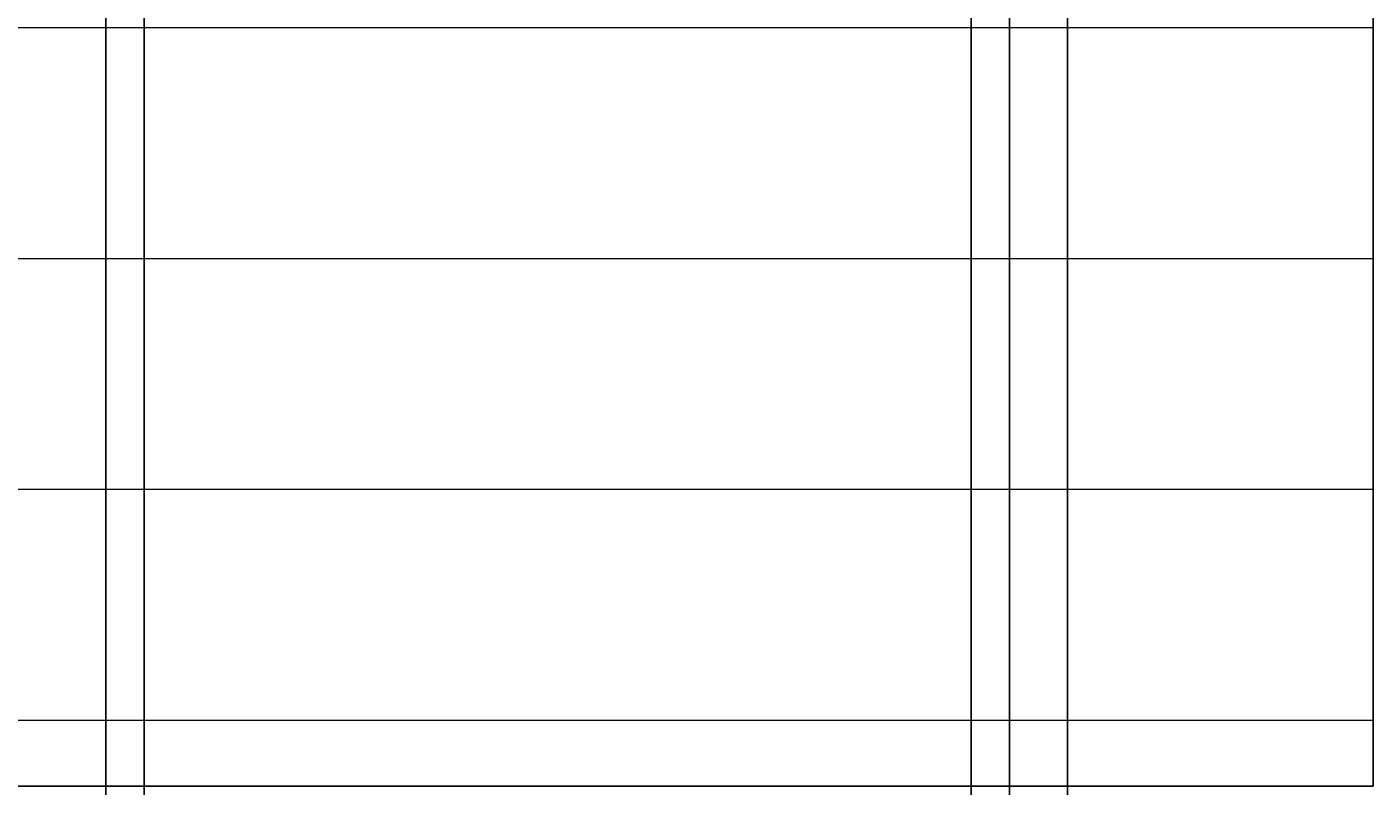
# Model space of a CAD drawing. Units: inches. Extents: x -6 to 289, y -8 to 323.
# Tile 31 of 107: x 209 to 244, y 10 to 30. Entities that reach past the tile are written whole.
import ezdxf

# ---------------------------------------------------------------- set-up
doc = ezdxf.new("R2010")
doc.units = ezdxf.units.IN
doc.header["$MEASUREMENT"] = 0
for name, color, linetype, lineweight in [('A-ANNO-DIMS', 2, 'Continuous', 18), ('A-DOOR', 3, 'Continuous', 25), ('A-ELEV-PATT', 8, 'Continuous', 13)]:
    doc.layers.add(name, color=color, linetype=linetype, lineweight=lineweight)
doc.styles.get("Standard").update_dxf_attribs({"font": 'arial.ttf'})
doc.dimstyles.get("Standard").update_dxf_attribs({"dimtxt": 0.18, "dimasz": 0.18, "dimexe": 0.18, "dimexo": 0.0625, "dimgap": 0.09, "dimtad": 0, "dimtih": 1, "dimtoh": 1, "dimdec": 4, "dimzin": 0, "dimdsep": 46, "dimtxsty": 'Standard', "dimcen": 0.09, "dimadec": 0, "dimazin": 0, "dimtfac": 1, "dimtdec": 4, "dimtofl": 0, "dimtmove": 0, "dimatfit": 3, "dimfxl": 1, "dimtolj": 1, "dimtzin": 0, "dimarcsym": 0})

# ---------------------------------------------------------------- blocks, each defined once
blk = doc.blocks.new('*D16')
at = {"layer": 'A-ANNO-DIMS', "color": 0, "lineweight": -2, "transparency": 16777216}
for p, q in [((9.943, 68.37), (9.943, -8.391)), ((272.973, 68.37), (272.973, -8.391)), ((10.123, -8.211), (140.993, -8.211)), ((272.793, -8.211), (141.923, -8.211))]:
    blk.add_line(p, q, dxfattribs=at)
at = {"layer": 'A-ANNO-DIMS', "color": 0, "transparency": 16777216}
for points in [[(10.123, -8.181), (10.123, -8.241), (9.943, -8.211)], [(272.793, -8.181), (272.793, -8.241), (272.973, -8.211)]]:
    blk.add_solid(points, dxfattribs=at)
at = {"layer": 'Defpoints', "color": 0, "transparency": 16777216}
for p in [(9.943, 68.432), (272.973, 68.432), (272.973, -8.211)]:
    blk.add_point(p, dxfattribs=at)
at = {"layer": 'A-ANNO-DIMS', "color": 0, "transparency": 16777216, "insert": (141.458, -8.211), "char_height": 0.18, "attachment_point": 5}
blk.add_mtext('\\A1;263.03', dxfattribs=at)
blk = doc.blocks.new('*D42')
at = {"layer": 'A-ANNO-DIMS', "color": 0, "lineweight": -2, "transparency": 16777216}
for p, q in [((190.792, 224.326), (190.792, -8.391)), ((211.292, 224.326), (211.292, -8.391)), ((190.972, -8.211), (200.716, -8.211)), ((211.112, -8.211), (201.368, -8.211))]:
    blk.add_line(p, q, dxfattribs=at)
at = {"layer": 'A-ANNO-DIMS', "color": 0, "transparency": 16777216}
for points in [[(190.972, -8.181), (190.972, -8.241), (190.792, -8.211)], [(211.112, -8.181), (211.112, -8.241), (211.292, -8.211)]]:
    blk.add_solid(points, dxfattribs=at)
at = {"layer": 'Defpoints', "color": 0, "transparency": 16777216}
for p in [(190.792, 224.389), (211.292, 224.389), (211.292, -8.211)]:
    blk.add_point(p, dxfattribs=at)
at = {"layer": 'A-ANNO-DIMS', "color": 0, "transparency": 16777216, "insert": (201.042, -8.211), "char_height": 0.18, "attachment_point": 5}
blk.add_mtext('\\A1;20.5', dxfattribs=at)
blk = doc.blocks.new('*D43')
at = {"layer": 'A-ANNO-DIMS', "color": 0, "lineweight": -2, "transparency": 16777216}
for p, q in [((211.292, 224.326), (211.292, -8.391)), ((212.292, 224.326), (212.292, -8.391)), ((211.472, -8.211), (211.669, -8.211)), ((212.112, -8.211), (211.915, -8.211))]:
    blk.add_line(p, q, dxfattribs=at)
at = {"layer": 'A-ANNO-DIMS', "color": 0, "transparency": 16777216}
for points in [[(211.472, -8.181), (211.472, -8.241), (211.292, -8.211)], [(212.112, -8.181), (212.112, -8.241), (212.292, -8.211)]]:
    blk.add_solid(points, dxfattribs=at)
at = {"layer": 'Defpoints', "color": 0, "transparency": 16777216}
for p in [(211.292, 224.389), (212.292, 224.389), (212.292, -8.211)]:
    blk.add_point(p, dxfattribs=at)
at = {"layer": 'A-ANNO-DIMS', "color": 0, "transparency": 16777216, "insert": (211.792, -8.211), "char_height": 0.18, "attachment_point": 5}
blk.add_mtext('\\A1;1', dxfattribs=at)
blk = doc.blocks.new('*D44')
at = {"layer": 'A-ANNO-DIMS', "color": 0, "lineweight": -2, "transparency": 16777216}
for p, q in [((212.292, 224.326), (212.292, -8.391)), ((233.792, 224.326), (233.792, -8.391)), ((212.472, -8.211), (222.716, -8.211)), ((233.612, -8.211), (223.368, -8.211))]:
    blk.add_line(p, q, dxfattribs=at)
at = {"layer": 'A-ANNO-DIMS', "color": 0, "transparency": 16777216}
for points in [[(212.472, -8.181), (212.472, -8.241), (212.292, -8.211)], [(233.612, -8.181), (233.612, -8.241), (233.792, -8.211)]]:
    blk.add_solid(points, dxfattribs=at)
at = {"layer": 'Defpoints', "color": 0, "transparency": 16777216}
for p in [(212.292, 224.389), (233.792, 224.389), (233.792, -8.211)]:
    blk.add_point(p, dxfattribs=at)
at = {"layer": 'A-ANNO-DIMS', "color": 0, "transparency": 16777216, "insert": (223.042, -8.211), "char_height": 0.18, "attachment_point": 5}
blk.add_mtext('\\A1;21.5', dxfattribs=at)
blk = doc.blocks.new('*D45')
at = {"layer": 'A-ANNO-DIMS', "color": 0, "lineweight": -2, "transparency": 16777216}
for p, q in [((234.792, 225.326), (234.792, -8.391)), ((233.792, 224.326), (233.792, -8.391)), ((233.972, -8.211), (234.169, -8.211)), ((234.612, -8.211), (234.415, -8.211))]:
    blk.add_line(p, q, dxfattribs=at)
at = {"layer": 'A-ANNO-DIMS', "color": 0, "transparency": 16777216}
for points in [[(233.972, -8.181), (233.972, -8.241), (233.792, -8.211)], [(234.612, -8.181), (234.612, -8.241), (234.792, -8.211)]]:
    blk.add_solid(points, dxfattribs=at)
at = {"layer": 'Defpoints', "color": 0, "transparency": 16777216}
for p in [(234.792, 225.389), (233.792, 224.389), (234.792, -8.211)]:
    blk.add_point(p, dxfattribs=at)
at = {"layer": 'A-ANNO-DIMS', "color": 0, "transparency": 16777216, "insert": (234.292, -8.211), "char_height": 0.18, "attachment_point": 5}
blk.add_mtext('\\A1;1', dxfattribs=at)
blk = doc.blocks.new('*D46')
at = {"layer": 'A-ANNO-DIMS', "color": 0, "lineweight": -2, "transparency": 16777216}
for p, q in [((236.292, 226.826), (236.292, -8.391)), ((234.792, 225.326), (234.792, -8.391)), ((234.972, -8.211), (235.296, -8.211)), ((236.112, -8.211), (235.788, -8.211))]:
    blk.add_line(p, q, dxfattribs=at)
at = {"layer": 'A-ANNO-DIMS', "color": 0, "transparency": 16777216}
for points in [[(234.972, -8.181), (234.972, -8.241), (234.792, -8.211)], [(236.112, -8.181), (236.112, -8.241), (236.292, -8.211)]]:
    blk.add_solid(points, dxfattribs=at)
at = {"layer": 'Defpoints', "color": 0, "transparency": 16777216}
for p in [(236.292, 226.889), (234.792, 225.389), (236.292, -8.211)]:
    blk.add_point(p, dxfattribs=at)
at = {"layer": 'A-ANNO-DIMS', "color": 0, "transparency": 16777216, "insert": (235.542, -8.211), "char_height": 0.18, "attachment_point": 5}
blk.add_mtext('\\A1;1.5', dxfattribs=at)

msp = doc.modelspace()

# ---------------------------------------------------------------- hatches: boundary and pattern name
at = {"layer": 'A-ELEV-PATT'}
h = msp.add_hatch(dxfattribs=at)
h.set_pattern_fill('_USER', color=256, scale=6, pattern_type=0)
h.set_pattern_definition([(0, (0, 0), (0, 6), [])])
h.paths.add_polyline_path([(184.1244, 48.0851), (124.008, 48.0851), (124.008, 10.2888), (184.1244, 10.2888)])
h.paths.add_polyline_path([(244.2408, 48.0851), (186.3604, 48.0851), (186.3604, 10.2888), (244.2408, 10.2888)])
h.paths.add_polyline_path([(208.2918, 114.2795), (190.7918, 114.2795), (190.7918, 71.2795), (208.2918, 71.2795)])
h.paths.add_polyline_path([(227.7918, 114.2795), (209.2918, 114.2795), (209.2918, 71.2795), (227.7918, 71.2795)])
h.paths.add_polyline_path([(211.2918, 224.3887), (190.7918, 224.3887), (190.7918, 162.3484), (211.2918, 162.3484)])
h.paths.add_polyline_path([(233.7918, 224.3887), (212.2918, 224.3887), (212.2918, 162.3484), (233.7918, 162.3484)])
h.paths.add_polyline_path([(166.3835, 224.154), (147.8835, 224.154), (147.8835, 181.154), (166.3835, 181.154)])
h.paths.add_polyline_path([(146.8835, 224.154), (129.3835, 224.154), (129.3835, 181.154), (146.8835, 181.154)])

# ---------------------------------------------------------------- linework, layer by layer
at = {"layer": 'A-DOOR'}
msp.add_lwpolyline([(124.008, 48.0851), (244.2408, 48.0851), (244.2408, 10.2888), (124.008, 10.2888)], close=True, dxfattribs=at)

# ---------------------------------------------------------------- dimensions: what is measured, and where the dimension line sits
at = {"layer": 'A-ANNO-DIMS'}
for base, p1, p2, override, picture, middle in [((236.2918, -8.2112), (234.7918, 225.3887), (236.2918, 226.8887), {"dimdec": 1, "dimlfac": 1, "dimrnd": 0, "dimzin": 0, "dimdsep": 46, "dimlunit": 2}, '*D46', (235.5418, -8.2112)), ((234.7918, -8.2112), (233.7918, 224.3887), (234.7918, 225.3887), {"dimdec": 0, "dimlfac": 1, "dimrnd": 0, "dimzin": 0, "dimdsep": 46, "dimlunit": 2}, '*D45', (234.2918, -8.2112)), ((211.2918, -8.2112), (190.7918, 224.3887), (211.2918, 224.3887), {"dimdec": 1, "dimlfac": 1, "dimrnd": 0, "dimzin": 0, "dimdsep": 46, "dimlunit": 2}, '*D42', (201.0418, -8.2112)), ((212.2918, -8.2112), (211.2918, 224.3887), (212.2918, 224.3887), {"dimdec": 0, "dimlfac": 1, "dimrnd": 0, "dimzin": 0, "dimdsep": 46, "dimlunit": 2}, '*D43', (211.7918, -8.2112)), ((233.7918, -8.2112), (212.2918, 224.3887), (233.7918, 224.3887), {"dimdec": 1, "dimlfac": 1, "dimrnd": 0, "dimzin": 0, "dimdsep": 46, "dimlunit": 2}, '*D44', (223.0418, -8.2112)), ((272.9733, -8.2112), (9.943, 68.4322), (272.9733, 68.4322), {"dimdec": 2, "dimlfac": 1, "dimrnd": 0, "dimzin": 0, "dimdsep": 46, "dimlunit": 2}, '*D16', (141.4581, -8.2112))]:
    dim = msp.add_linear_dim(base=base, p1=p1, p2=p2, dimstyle='Standard', override=override, dxfattribs=at)
    dim.commit()
    dim.dimension.update_dxf_attribs({"geometry": picture, "text_midpoint": middle})

doc.saveas('drawing.dxf')
